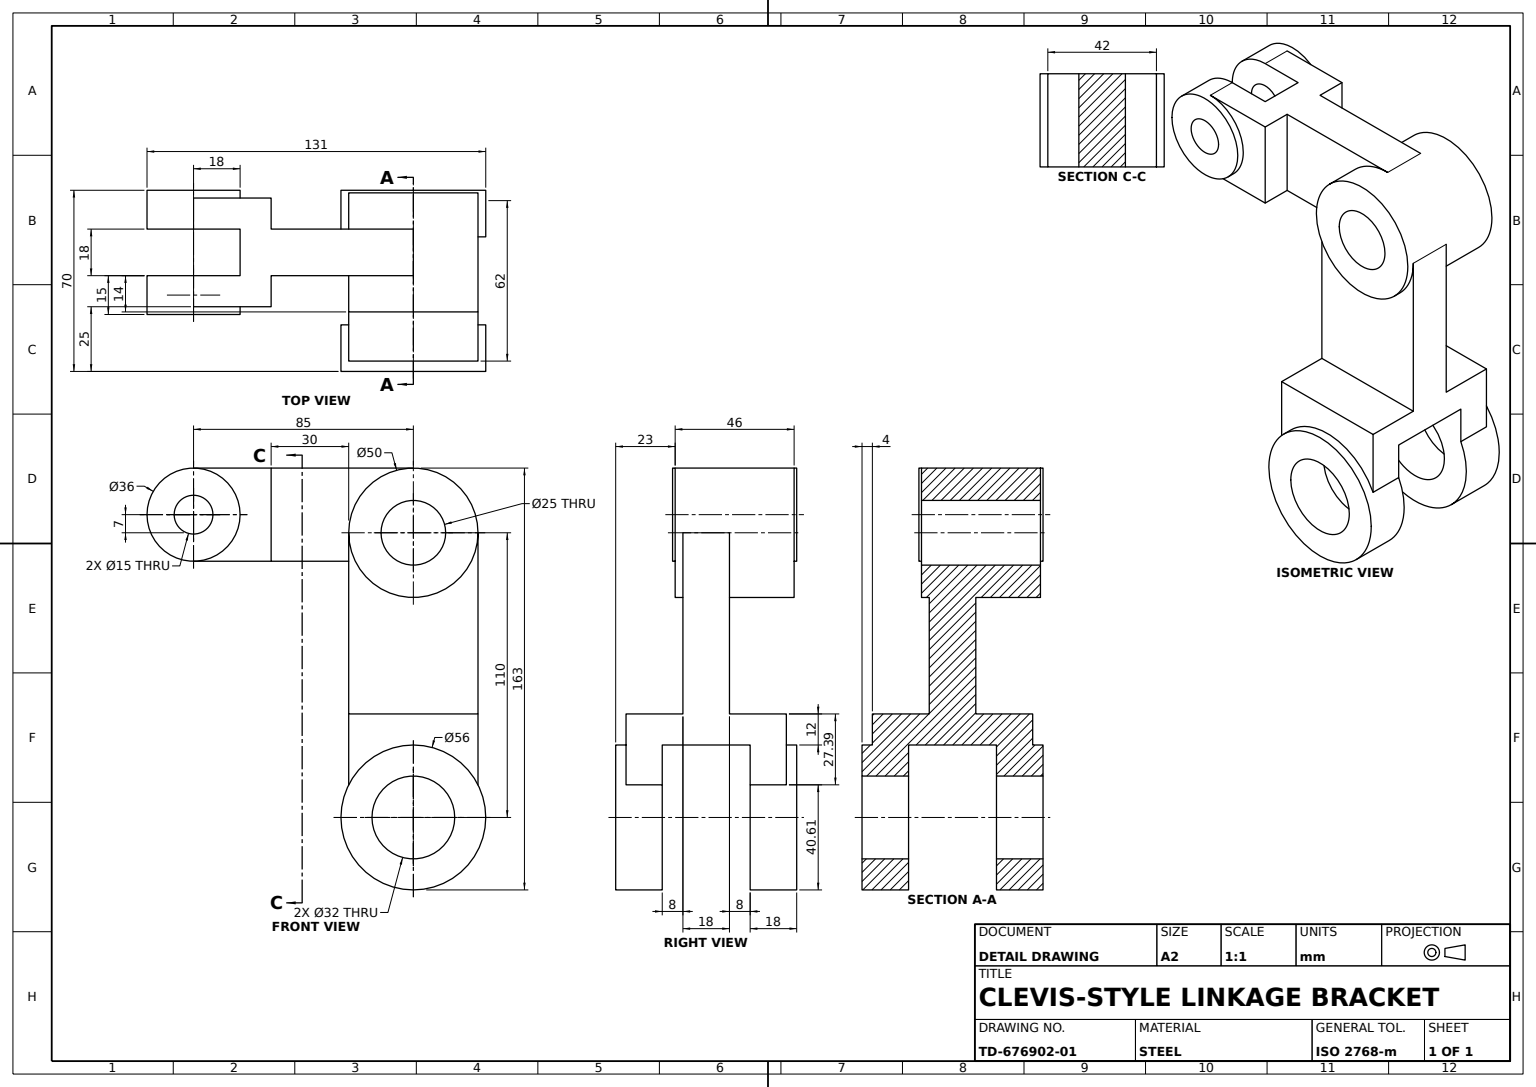
SolidWorks part; units mm, degrees
material "Plain Carbon Steel"
ref_plane "Front Plane" through (0, 0, 0) normal (0, 0, 1) x (1, 0, 0)
ref_plane "Top Plane" through (0, 0, 0) normal (0, 1, 0) x (1, 0, 0)
ref_plane "Right Plane" through (0, 0, 0) normal (1, 0, 0) x (0, 0, -1)
sketch "Lower Hub A Sketch" plane through (0, 0, 0) normal (1, 0, 0) x (0, 0, -1)
  circle A0 centre (0, 0) radius 28
  dimension "D1" = 56
extrude "Lower Hub A Ø56" add sketch "Lower Hub A Sketch" against normal blind 18
ref_plane "Lower Hub B Plane" through (-52, 0, 0) normal (-1, 0, 0) x (0, 0, 1)
sketch "Lower Hub B Sketch" plane through (-52, 0, 0) normal (-1, 0, 0) x (0, 0, 1)
  circle A0 centre (0, 0) radius 28
  dimension "D1" = 56
extrude "Lower Hub B Ø56" add sketch "Lower Hub B Sketch" along normal blind 18 separate body
sketch "Lower Fork Block Sketch" plane through (-18, 0, 0) normal (-1, 0, 0) x (0, 0, 1)
  line L1 (0, 40) -> (25, 40)
  line L2 (25, 40) -> (25, 12.6095)
  line L3 (0, 40) -> (-25, 40)
  line L4 (-25, 40) -> (-25, 12.6095)
  arc A1 (25, 12.6095) -> (-25, 12.6095) centre (0, 0) ccw
  point P0 (0, 28)
  dimension "D5" = 28
  dimension "D1" = 50
  dimension "D2" = 27.3905
  dimension "D3" = 12
  dimension "D4" = 27.3905
extrude "Lower Fork Block" add sketch "Lower Fork Block Sketch" along normal blind 48 and the other way blind 14
sketch "Lower Fork Slot Sketch" plane through (0, 0, 25) normal (0, 0, 1) x (1, 0, 0)
  line L2 (-52, 28) -> (-18, 28)
  line L3 (-18, 28) -> (-18, 12.6095)
  line L4 (-18, 12.6095) -> (-52, 12.6095)
  line L5 (-52, 12.6095) -> (-52, 28)
  dimension "D1" = 15.3905
extrude "Lower Fork Slot" cut sketch "Lower Fork Slot Sketch" against normal blind 65
sketch "Vertical Arm Sketch" plane through (0, 0, 25) normal (0, 0, 1) x (1, 0, 0)
  line L0 (-35, 40) -> (-26, 40)
  line L1 (-4, 40) -> (-66, 40) construction
  line L2 (-35, 40) -> (-44, 40)
  line L4 (-26, 40) -> (-26, 110)
  line L5 (-26, 110) -> (-44, 110)
  line L6 (-44, 110) -> (-44, 40)
  dimension "D1" = 18
  dimension "D2" = 70
  dimension "D3" = 44
extrude "Vertical Arm" add sketch "Vertical Arm Sketch" against normal blind 50
sketch "Upper Hub Sketch" plane through (-26, 0, 0) normal (1, 0, 0) x (0, 0, -1)
  line L0 (25, 110) -> (-25, 110) construction
  circle A0 centre (0, 110) radius 25
extrude "Upper Hub" add sketch "Upper Hub Sketch" along normal blind 3 and the other way blind 43
ref_plane "Upper Fork Arm Plane" through (0, 135, 0) normal (0, 1, 0) x (1, 0, 0)
sketch "Upper Fork Arm Sketch" plane through (0, 135, 0) normal (0, 1, 0) x (1, 0, 0)
  line L2 (-37, 0) -> (-37, -55)
  line L3 (-37, -55) -> (-25, -55)
  line L4 (-25, -55) -> (-25, -85)
  line L5 (-25, -85) -> (-37, -85)
  line L6 (-37, -85) -> (-37, -67)
  line L7 (-37, -67) -> (-55, -67)
  line L8 (-55, -67) -> (-55, -85)
  line L9 (-55, -85) -> (-67, -85)
  line L10 (-67, -85) -> (-67, -55)
  line L11 (-67, -55) -> (-55, -55)
  line L12 (-55, -55) -> (-55, 0)
  line L13 (-55, 0) -> (-37, 0)
  dimension "D1" = 18
  dimension "D2" = 30
  dimension "D3" = 30
  dimension "D4" = 18
  dimension "D5" = 55
  dimension "D6" = 85
  dimension "D7" = 67
  dimension "D8" = 42
  dimension "D9" = 25
  dimension "D10" = 30
  dimension "D11" = 12
extrude "Upper Fork Arm" add sketch "Upper Fork Arm Sketch" against normal blind 36
sketch "Fork Eye A Sketch" plane through (-55, 0, 0) normal (1, 0, 0) x (0, 0, -1)
  line L0 (-85, 99) -> (-85, 135) construction
  circle A0 centre (-85, 117) radius 18
  dimension "D1" = 36
extrude "Fork Eye A Ø36" add sketch "Fork Eye A Sketch" against normal blind 15
sketch "Fork Eye B Sketch" plane through (-37, 0, 0) normal (-1, 0, 0) x (0, 0, 1)
  circle A0 centre (85, 117) radius 18
extrude "Fork Eye B" add sketch "Fork Eye B Sketch" against normal blind 15
sketch "Lower Pivot Bore Sketch" plane through (0, 0, 0) normal (1, 0, 0) x (0, 0, -1)
  circle A0 centre (0, 0) radius 16
  dimension "D1" = 32
extrude "Lower Pivot Bore Ø32" cut sketch "Lower Pivot Bore Sketch" against normal blind 132
sketch "Upper Hub Bore Sketch" plane through (-69, 0, 0) normal (-1, 0, 0) x (0, 0, 1)
  circle A0 centre (0, 110) radius 12.5
  dimension "D1" = 25
extrude "Upper Hub Bore Ø25" cut sketch "Upper Hub Bore Sketch" against normal blind 132
sketch "Fork Eye Bore Sketch" plane through (-70, 0, 0) normal (-1, 0, 0) x (0, 0, 1)
  circle A0 centre (85, 117) radius 7.5
  dimension "D1" = 15
extrude "Fork Eye Bore Ø15" cut sketch "Fork Eye Bore Sketch" against normal blind 132
